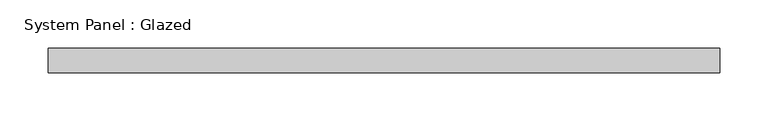
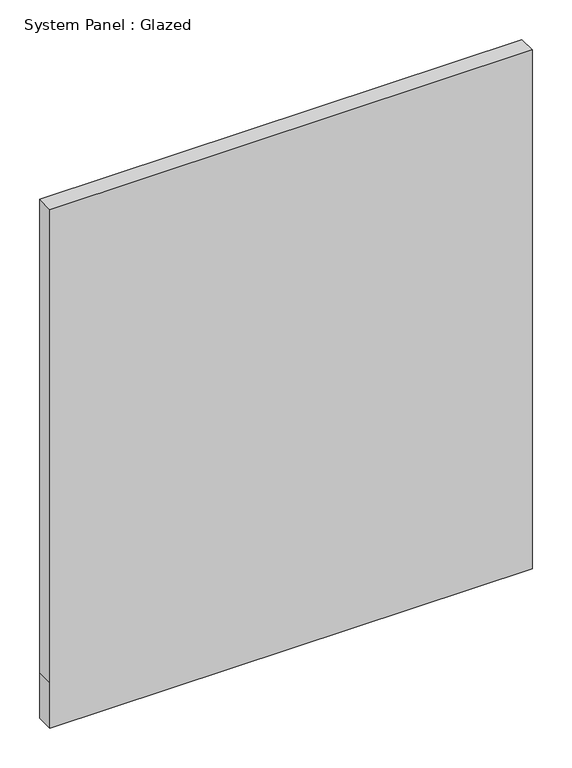
"""IFC4 building model written with IfcOpenShell, lengths in millimetres: plate geometry, System Panel : Glazed."""

from ifc_helpers import new_model, si_unit, frame, origin, place, context, project, spatial, polyline, outline, extrude, source, transform, mapped, element, save


def system_panel_glazed_ee93d072(model_context):
    return source(origin(), model_context, "Body", "SweptSolid", [
        extrude(outline(polyline([(0.0, -349.25), (0.0, 349.25), (69.85, 349.25), (794.4489237, 349.25), (794.4489237, -349.25), (69.85, -349.25), (0.0, -349.25)])), frame((0.0, 19.05, 0.0), z_axis=(0.0, 1.0, 0.0), x_axis=(0.0, 0.0, 1.0)), (0.0, 0.0, 1.0), 25.4),
    ])


if __name__ == "__main__":
    model = new_model("IFC4")
    model_context = context("Model", 3, world=origin())
    ifc_project = project(units=[si_unit("LENGTHUNIT", "METRE", prefix="MILLI")], contexts=[model_context])
    site = spatial("IfcSite", under=ifc_project)
    building = spatial("IfcBuilding", under=site)
    placement = place(None, origin())
    system_panel_glazed_shape = system_panel_glazed_ee93d072(model_context)
    element("IfcPlate", 1, ObjectType="System Panel : Glazed", at=placement, inside=building, context=model_context, shape_type="MappedRepresentation", body=[
        mapped(system_panel_glazed_shape, transform((0.0, 0.0, 0.0), x_axis=(1.0, 0.0, 0.0), y_axis=(0.0, 1.0, 0.0), z_axis=(0.0, 0.0, 1.0))),
    ])
    save(model, "model.ifc")

# Revit data of these elements
# Type "System Panel : Glazed"
#   Construction Type Id = "GSP4R"
#   Analytic Construction = "1/8 in Pilkington single glazing"
#   Visual Light Transmittance = 0.9
#   Solar Heat Gain Coefficient = 0.86
#   Heat Transfer Coefficient (U) = 1.18115 BTU/(h·ft²·°F)
#   Define Thermal Properties by = 1
# Element 1 (IfcPlate, "System Panel : Glazed")
#   Materials on its faces: "Glass"
# Materials
#   "Glass": class "Glass", colour RGB 0 128 192, transparency 0.75, Description = "Soda Lime Glass", Cost = 0
